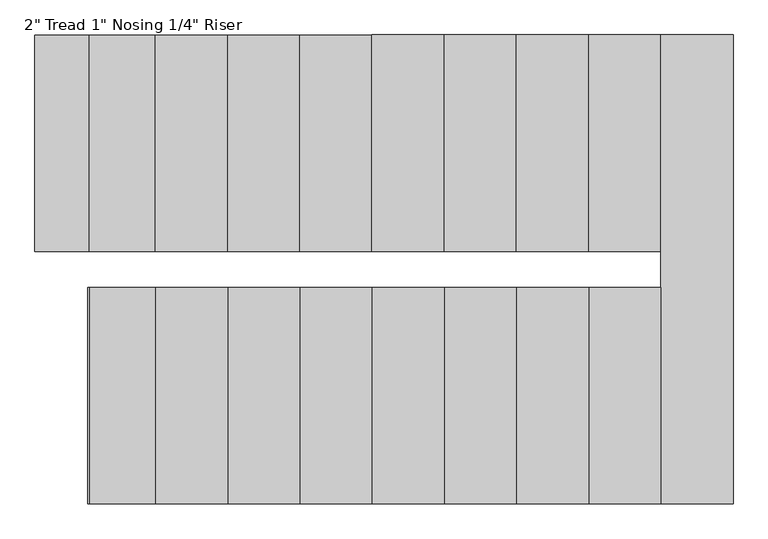
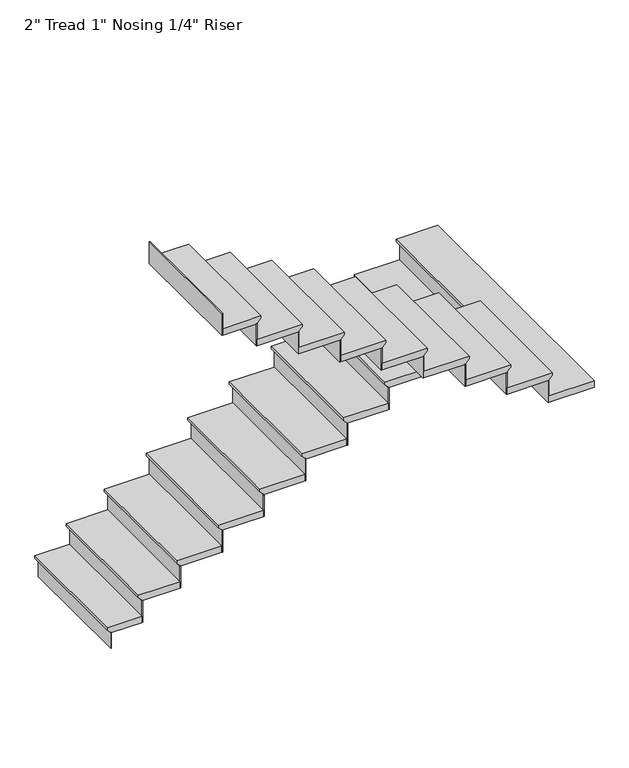
"""IFC4 building model written with IfcOpenShell, lengths in millimetres: stair flight geometry."""

from ifc_helpers import new_model, si_unit, origin, place, context, project, spatial, faceted_brep, source, transform, mapped, element, save


def stair_flight_fa6bf0c5(model_context):
    return source(origin(), model_context, "Body", "Brep", [
        faceted_brep([(8572.5, 8280.4, 150.2833333), (8572.5, 8280.4, 169.3333333), (8572.5, 9194.8, 169.3333333), (8572.5, 9194.8, 150.2833333), (8597.9, 8280.4, 124.8833333), (8597.9, 9194.8, 124.8833333), (8826.5, 8280.4, 169.3333333), (8826.5, 9194.8, 169.3333333), (8597.9, 9194.8, 118.5333333), (8826.5, 9194.8, 118.5333333), (8826.5, 8280.4, 118.5333333), (8597.9, 8280.4, 118.5333333)], [[[0, 1, 2, 3]], [[4, 0, 3, 5]], [[2, 1, 6, 7]], [[8, 9, 10, 11]], [[2, 7, 9, 8, 5, 3]], [[8, 11, 4, 5]], [[6, 1, 0, 4, 11, 10]], [[7, 6, 10, 9]]]),
        faceted_brep([(8597.9, 8280.4, 118.5333333), (8597.9, 8280.4, 0.0), (8604.25, 8280.4, 0.0), (8604.25, 8280.4, 118.5333333), (8597.9, 9194.8, 118.5333333), (8604.25, 9194.8, 118.5333333), (8604.25, 9194.8, 0.0), (8597.9, 9194.8, 0.0)], [[[0, 1, 2, 3]], [[4, 5, 6, 7]], [[1, 0, 4, 7]], [[2, 1, 7, 6]], [[3, 2, 6, 5]], [[0, 3, 5, 4]]]),
        faceted_brep([(8826.5, 8280.4, 287.8666667), (8826.5, 8280.4, 118.5333333), (8832.85, 8280.4, 118.5333333), (8832.85, 8280.4, 287.8666667), (8826.5, 9194.8, 287.8666667), (8832.85, 9194.8, 287.8666667), (8832.85, 9194.8, 118.5333333), (8826.5, 9194.8, 118.5333333)], [[[0, 1, 2, 3]], [[4, 5, 6, 7]], [[1, 0, 4, 7]], [[2, 1, 7, 6]], [[3, 2, 6, 5]], [[0, 3, 5, 4]]]),
        faceted_brep([(8801.1, 9194.8, 338.6666667), (8801.1, 8280.4, 338.6666667), (9105.9, 8280.4, 338.6666667), (9105.9, 9194.8, 338.6666667), (8826.5, 9194.8, 287.8666667), (9105.9, 9194.8, 287.8666667), (9105.9, 8280.4, 287.8666667), (8826.5, 8280.4, 287.8666667), (8826.5, 9194.8, 294.2166667), (8801.1, 9194.8, 319.6166667), (8826.5, 8280.4, 294.2166667), (8801.1, 8280.4, 319.6166667)], [[[0, 1, 2, 3]], [[4, 5, 6, 7]], [[0, 3, 5, 4, 8, 9]], [[4, 7, 10, 8]], [[2, 1, 11, 10, 7, 6]], [[3, 2, 6, 5]], [[11, 1, 0, 9]], [[10, 11, 9, 8]]]),
        faceted_brep([(9105.9, 8280.4, 457.2), (9105.9, 8280.4, 287.8666667), (9112.25, 8280.4, 287.8666667), (9112.25, 8280.4, 457.2), (9105.9, 9194.8, 457.2), (9112.25, 9194.8, 457.2), (9112.25, 9194.8, 287.8666667), (9105.9, 9194.8, 287.8666667)], [[[0, 1, 2, 3]], [[4, 5, 6, 7]], [[1, 0, 4, 7]], [[2, 1, 7, 6]], [[3, 2, 6, 5]], [[0, 3, 5, 4]]]),
        faceted_brep([(9080.5, 9194.8, 508.0), (9080.5, 8280.4, 508.0), (9410.7, 8280.4, 508.0), (9410.7, 9194.8, 508.0), (9105.9, 9194.8, 457.2), (9410.7, 9194.8, 457.2), (9410.7, 8280.4, 457.2), (9105.9, 8280.4, 457.2), (9105.9, 9194.8, 463.55), (9080.5, 9194.8, 488.95), (9105.9, 8280.4, 463.55), (9080.5, 8280.4, 488.95)], [[[0, 1, 2, 3]], [[4, 5, 6, 7]], [[0, 3, 5, 4, 8, 9]], [[4, 7, 10, 8]], [[2, 1, 11, 10, 7, 6]], [[3, 2, 6, 5]], [[11, 1, 0, 9]], [[10, 11, 9, 8]]]),
        faceted_brep([(9410.7, 8280.4, 626.5333333), (9410.7, 8280.4, 457.2), (9417.05, 8280.4, 457.2), (9417.05, 8280.4, 626.5333333), (9410.7, 9194.8, 626.5333333), (9417.05, 9194.8, 626.5333333), (9417.05, 9194.8, 457.2), (9410.7, 9194.8, 457.2)], [[[0, 1, 2, 3]], [[4, 5, 6, 7]], [[1, 0, 4, 7]], [[2, 1, 7, 6]], [[3, 2, 6, 5]], [[0, 3, 5, 4]]]),
        faceted_brep([(9385.3, 9194.8, 677.3333333), (9385.3, 8280.4, 677.3333333), (9715.5, 8280.4, 677.3333333), (9715.5, 9194.8, 677.3333333), (9410.7, 9194.8, 626.5333333), (9715.5, 9194.8, 626.5333333), (9715.5, 8280.4, 626.5333333), (9410.7, 8280.4, 626.5333333), (9410.7, 9194.8, 632.8833333), (9385.3, 9194.8, 658.2833333), (9410.7, 8280.4, 632.8833333), (9385.3, 8280.4, 658.2833333)], [[[0, 1, 2, 3]], [[4, 5, 6, 7]], [[0, 3, 5, 4, 8, 9]], [[4, 7, 10, 8]], [[2, 1, 11, 10, 7, 6]], [[3, 2, 6, 5]], [[11, 1, 0, 9]], [[10, 11, 9, 8]]]),
        faceted_brep([(9715.5, 8280.4, 795.8666667), (9715.5, 8280.4, 626.5333333), (9721.85, 8280.4, 626.5333333), (9721.85, 8280.4, 795.8666667), (9715.5, 9194.8, 795.8666667), (9721.85, 9194.8, 795.8666667), (9721.85, 9194.8, 626.5333333), (9715.5, 9194.8, 626.5333333)], [[[0, 1, 2, 3]], [[4, 5, 6, 7]], [[1, 0, 4, 7]], [[2, 1, 7, 6]], [[3, 2, 6, 5]], [[0, 3, 5, 4]]]),
        faceted_brep([(9690.1, 9194.8, 846.6666667), (9690.1, 8280.4, 846.6666667), (10020.3, 8280.4, 846.6666667), (10020.3, 9194.8, 846.6666667), (9715.5, 9194.8, 795.8666667), (10020.3, 9194.8, 795.8666667), (10020.3, 8280.4, 795.8666667), (9715.5, 8280.4, 795.8666667), (9715.5, 9194.8, 802.2166667), (9690.1, 9194.8, 827.6166667), (9715.5, 8280.4, 802.2166667), (9690.1, 8280.4, 827.6166667)], [[[0, 1, 2, 3]], [[4, 5, 6, 7]], [[0, 3, 5, 4, 8, 9]], [[4, 7, 10, 8]], [[2, 1, 11, 10, 7, 6]], [[3, 2, 6, 5]], [[11, 1, 0, 9]], [[10, 11, 9, 8]]]),
        faceted_brep([(10020.3, 8280.4, 965.2), (10020.3, 8280.4, 795.8666667), (10026.65, 8280.4, 795.8666667), (10026.65, 8280.4, 965.2), (10020.3, 9194.8, 965.2), (10026.65, 9194.8, 965.2), (10026.65, 9194.8, 795.8666667), (10020.3, 9194.8, 795.8666667)], [[[0, 1, 2, 3]], [[4, 5, 6, 7]], [[1, 0, 4, 7]], [[2, 1, 7, 6]], [[3, 2, 6, 5]], [[0, 3, 5, 4]]]),
        faceted_brep([(9994.9, 9194.8, 1016.0), (9994.9, 8280.4, 1016.0), (10325.1, 8280.4, 1016.0), (10325.1, 9194.8, 1016.0), (10020.3, 9194.8, 965.2), (10325.1, 9194.8, 965.2), (10325.1, 8280.4, 965.2), (10020.3, 8280.4, 965.2), (10020.3, 9194.8, 971.55), (9994.9, 9194.8, 996.95), (10020.3, 8280.4, 971.55), (9994.9, 8280.4, 996.95)], [[[0, 1, 2, 3]], [[4, 5, 6, 7]], [[0, 3, 5, 4, 8, 9]], [[4, 7, 10, 8]], [[2, 1, 11, 10, 7, 6]], [[3, 2, 6, 5]], [[11, 1, 0, 9]], [[10, 11, 9, 8]]]),
        faceted_brep([(10325.1, 8280.4, 1134.5333333), (10325.1, 8280.4, 965.2), (10331.45, 8280.4, 965.2), (10331.45, 8280.4, 1134.5333333), (10325.1, 9194.8, 1134.5333333), (10331.45, 9194.8, 1134.5333333), (10331.45, 9194.8, 965.2), (10325.1, 9194.8, 965.2)], [[[0, 1, 2, 3]], [[4, 5, 6, 7]], [[1, 0, 4, 7]], [[2, 1, 7, 6]], [[3, 2, 6, 5]], [[0, 3, 5, 4]]]),
        faceted_brep([(10299.7, 9194.8, 1185.3333333), (10299.7, 8280.4, 1185.3333333), (10629.9, 8280.4, 1185.3333333), (10629.9, 9194.8, 1185.3333333), (10325.1, 9194.8, 1134.5333333), (10629.9, 9194.8, 1134.5333333), (10629.9, 8280.4, 1134.5333333), (10325.1, 8280.4, 1134.5333333), (10325.1, 9194.8, 1140.8833333), (10299.7, 9194.8, 1166.2833333), (10325.1, 8280.4, 1140.8833333), (10299.7, 8280.4, 1166.2833333)], [[[0, 1, 2, 3]], [[4, 5, 6, 7]], [[0, 3, 5, 4, 8, 9]], [[4, 7, 10, 8]], [[2, 1, 11, 10, 7, 6]], [[3, 2, 6, 5]], [[11, 1, 0, 9]], [[10, 11, 9, 8]]]),
        faceted_brep([(10629.9, 8280.4, 1303.8666667), (10629.9, 8280.4, 1134.5333333), (10636.25, 8280.4, 1134.5333333), (10636.25, 8280.4, 1303.8666667), (10629.9, 9194.8, 1303.8666667), (10636.25, 9194.8, 1303.8666667), (10636.25, 9194.8, 1134.5333333), (10629.9, 9194.8, 1134.5333333)], [[[0, 1, 2, 3]], [[4, 5, 6, 7]], [[1, 0, 4, 7]], [[2, 1, 7, 6]], [[3, 2, 6, 5]], [[0, 3, 5, 4]]]),
        faceted_brep([(10604.5, 9194.8, 1354.6666667), (10604.5, 8280.4, 1354.6666667), (10934.7, 8280.4, 1354.6666667), (10934.7, 9194.8, 1354.6666667), (10629.9, 9194.8, 1303.8666667), (10934.7, 9194.8, 1303.8666667), (10934.7, 8280.4, 1303.8666667), (10629.9, 8280.4, 1303.8666667), (10629.9, 9194.8, 1310.2166667), (10604.5, 9194.8, 1335.6166667), (10629.9, 8280.4, 1310.2166667), (10604.5, 8280.4, 1335.6166667)], [[[0, 1, 2, 3]], [[4, 5, 6, 7]], [[0, 3, 5, 4, 8, 9]], [[4, 7, 10, 8]], [[2, 1, 11, 10, 7, 6]], [[3, 2, 6, 5]], [[11, 1, 0, 9]], [[10, 11, 9, 8]]]),
        faceted_brep([(10934.7, 8280.4, 1473.2), (10934.7, 8280.4, 1303.8666667), (10941.05, 8280.4, 1303.8666667), (10941.05, 8280.4, 1473.2), (10934.7, 9194.8, 1473.2), (10941.05, 9194.8, 1473.2), (10941.05, 9194.8, 1303.8666667), (10934.7, 9194.8, 1303.8666667)], [[[0, 1, 2, 3]], [[4, 5, 6, 7]], [[1, 0, 4, 7]], [[2, 1, 7, 6]], [[3, 2, 6, 5]], [[0, 3, 5, 4]]]),
        faceted_brep([(10909.3, 9194.8, 1524.0), (10909.3, 8280.4, 1524.0), (11239.5, 8280.4, 1524.0), (11239.5, 9194.8, 1524.0), (10934.7, 9194.8, 1473.2), (11239.5, 9194.8, 1473.2), (11239.5, 8280.4, 1473.2), (10934.7, 8280.4, 1473.2), (10934.7, 9194.8, 1479.55), (10909.3, 9194.8, 1504.95), (10934.7, 8280.4, 1479.55), (10909.3, 8280.4, 1504.95)], [[[0, 1, 2, 3]], [[4, 5, 6, 7]], [[0, 3, 5, 4, 8, 9]], [[4, 7, 10, 8]], [[2, 1, 11, 10, 7, 6]], [[3, 2, 6, 5]], [[11, 1, 0, 9]], [[10, 11, 9, 8]]]),
        faceted_brep([(11239.5, 8280.4, 1642.5333333), (11239.5, 8280.4, 1473.2), (11245.85, 8280.4, 1473.2), (11245.85, 8280.4, 1642.5333333), (11239.5, 9194.8, 1642.5333333), (11245.85, 9194.8, 1642.5333333), (11245.85, 9194.8, 1473.2), (11239.5, 9194.8, 1473.2)], [[[0, 1, 2, 3]], [[4, 5, 6, 7]], [[1, 0, 4, 7]], [[2, 1, 7, 6]], [[3, 2, 6, 5]], [[0, 3, 5, 4]]]),
        faceted_brep([(11188.7, 7213.6, 1693.3333333), (11518.9, 7213.6, 1693.3333333), (11518.9, 9194.8, 1693.3333333), (11214.1, 9194.8, 1693.3333333), (11214.1, 8128.0, 1693.3333333), (11188.7, 8128.0, 1693.3333333), (11518.9, 7213.6, 1642.5333333), (11188.7, 7213.6, 1642.5333333), (11188.7, 8128.0, 1642.5333333), (11214.1, 8128.0, 1642.5333333), (11214.1, 8280.4, 1642.5333333), (11239.5, 8280.4, 1642.5333333), (11239.5, 9194.8, 1642.5333333), (11518.9, 9194.8, 1642.5333333), (11239.5, 9194.8, 1648.8833333), (11214.1, 9194.8, 1674.2833333), (11239.5, 8280.4, 1648.8833333), (11214.1, 8280.4, 1674.2833333)], [[[0, 1, 2, 3, 4, 5]], [[6, 7, 8, 9, 10, 11, 12, 13]], [[1, 0, 7, 6]], [[2, 1, 6, 13]], [[3, 2, 13, 12, 14, 15]], [[12, 11, 16, 14]], [[11, 10, 17, 16]], [[4, 3, 15, 17, 10, 9]], [[5, 4, 9, 8]], [[0, 5, 8, 7]], [[15, 14, 16, 17]]]),
        faceted_brep([(11188.7, 8128.0, 1811.8666667), (11188.7, 8128.0, 1642.5333333), (11182.35, 8128.0, 1642.5333333), (11182.35, 8128.0, 1811.8666667), (11188.7, 7213.6, 1811.8666667), (11182.35, 7213.6, 1811.8666667), (11182.35, 7213.6, 1642.5333333), (11188.7, 7213.6, 1642.5333333)], [[[0, 1, 2, 3]], [[4, 5, 6, 7]], [[1, 0, 4, 7]], [[2, 1, 7, 6]], [[3, 2, 6, 5]], [[0, 3, 5, 4]]]),
        faceted_brep([(11214.1, 7213.6, 1862.6666667), (11214.1, 8128.0, 1862.6666667), (10883.9, 8128.0, 1862.6666667), (10883.9, 7213.6, 1862.6666667), (11188.7, 7213.6, 1811.8666667), (10883.9, 7213.6, 1811.8666667), (10883.9, 8128.0, 1811.8666667), (11188.7, 8128.0, 1811.8666667), (11188.7, 7213.6, 1818.2166667), (11214.1, 7213.6, 1843.6166667), (11188.7, 8128.0, 1818.2166667), (11214.1, 8128.0, 1843.6166667)], [[[0, 1, 2, 3]], [[4, 5, 6, 7]], [[0, 3, 5, 4, 8, 9]], [[4, 7, 10, 8]], [[2, 1, 11, 10, 7, 6]], [[3, 2, 6, 5]], [[11, 1, 0, 9]], [[10, 11, 9, 8]]]),
        faceted_brep([(10883.9, 8128.0, 1981.2), (10883.9, 8128.0, 1811.8666667), (10877.55, 8128.0, 1811.8666667), (10877.55, 8128.0, 1981.2), (10883.9, 7213.6, 1981.2), (10877.55, 7213.6, 1981.2), (10877.55, 7213.6, 1811.8666667), (10883.9, 7213.6, 1811.8666667)], [[[0, 1, 2, 3]], [[4, 5, 6, 7]], [[1, 0, 4, 7]], [[2, 1, 7, 6]], [[3, 2, 6, 5]], [[0, 3, 5, 4]]]),
        faceted_brep([(10909.3, 7213.6, 2032.0), (10909.3, 8128.0, 2032.0), (10579.1, 8128.0, 2032.0), (10579.1, 7213.6, 2032.0), (10883.9, 7213.6, 1981.2), (10579.1, 7213.6, 1981.2), (10579.1, 8128.0, 1981.2), (10883.9, 8128.0, 1981.2), (10883.9, 7213.6, 1987.55), (10909.3, 7213.6, 2012.95), (10883.9, 8128.0, 1987.55), (10909.3, 8128.0, 2012.95)], [[[0, 1, 2, 3]], [[4, 5, 6, 7]], [[0, 3, 5, 4, 8, 9]], [[4, 7, 10, 8]], [[2, 1, 11, 10, 7, 6]], [[3, 2, 6, 5]], [[11, 1, 0, 9]], [[10, 11, 9, 8]]]),
        faceted_brep([(10579.1, 8128.0, 2150.5333333), (10579.1, 8128.0, 1981.2), (10572.75, 8128.0, 1981.2), (10572.75, 8128.0, 2150.5333333), (10579.1, 7213.6, 2150.5333333), (10572.75, 7213.6, 2150.5333333), (10572.75, 7213.6, 1981.2), (10579.1, 7213.6, 1981.2)], [[[0, 1, 2, 3]], [[4, 5, 6, 7]], [[1, 0, 4, 7]], [[2, 1, 7, 6]], [[3, 2, 6, 5]], [[0, 3, 5, 4]]]),
        faceted_brep([(10604.5, 7213.6, 2201.3333333), (10604.5, 8128.0, 2201.3333333), (10274.3, 8128.0, 2201.3333333), (10274.3, 7213.6, 2201.3333333), (10579.1, 7213.6, 2150.5333333), (10274.3, 7213.6, 2150.5333333), (10274.3, 8128.0, 2150.5333333), (10579.1, 8128.0, 2150.5333333), (10579.1, 7213.6, 2156.8833333), (10604.5, 7213.6, 2182.2833333), (10579.1, 8128.0, 2156.8833333), (10604.5, 8128.0, 2182.2833333)], [[[0, 1, 2, 3]], [[4, 5, 6, 7]], [[0, 3, 5, 4, 8, 9]], [[4, 7, 10, 8]], [[2, 1, 11, 10, 7, 6]], [[3, 2, 6, 5]], [[11, 1, 0, 9]], [[10, 11, 9, 8]]]),
        faceted_brep([(10274.3, 8128.0, 2319.8666667), (10274.3, 8128.0, 2150.5333333), (10267.95, 8128.0, 2150.5333333), (10267.95, 8128.0, 2319.8666667), (10274.3, 7213.6, 2319.8666667), (10267.95, 7213.6, 2319.8666667), (10267.95, 7213.6, 2150.5333333), (10274.3, 7213.6, 2150.5333333)], [[[0, 1, 2, 3]], [[4, 5, 6, 7]], [[1, 0, 4, 7]], [[2, 1, 7, 6]], [[3, 2, 6, 5]], [[0, 3, 5, 4]]]),
        faceted_brep([(10299.7, 7213.6, 2370.6666667), (10299.7, 8128.0, 2370.6666667), (9969.5, 8128.0, 2370.6666667), (9969.5, 7213.6, 2370.6666667), (10274.3, 7213.6, 2319.8666667), (9969.5, 7213.6, 2319.8666667), (9969.5, 8128.0, 2319.8666667), (10274.3, 8128.0, 2319.8666667), (10274.3, 7213.6, 2326.2166667), (10299.7, 7213.6, 2351.6166667), (10274.3, 8128.0, 2326.2166667), (10299.7, 8128.0, 2351.6166667)], [[[0, 1, 2, 3]], [[4, 5, 6, 7]], [[0, 3, 5, 4, 8, 9]], [[4, 7, 10, 8]], [[2, 1, 11, 10, 7, 6]], [[3, 2, 6, 5]], [[11, 1, 0, 9]], [[10, 11, 9, 8]]]),
        faceted_brep([(9969.5, 8128.0, 2489.2), (9969.5, 8128.0, 2319.8666667), (9963.15, 8128.0, 2319.8666667), (9963.15, 8128.0, 2489.2), (9969.5, 7213.6, 2489.2), (9963.15, 7213.6, 2489.2), (9963.15, 7213.6, 2319.8666667), (9969.5, 7213.6, 2319.8666667)], [[[0, 1, 2, 3]], [[4, 5, 6, 7]], [[1, 0, 4, 7]], [[2, 1, 7, 6]], [[3, 2, 6, 5]], [[0, 3, 5, 4]]]),
        faceted_brep([(9994.9, 7213.6, 2540.0), (9994.9, 8128.0, 2540.0), (9664.7, 8128.0, 2540.0), (9664.7, 7213.6, 2540.0), (9969.5, 7213.6, 2489.2), (9664.7, 7213.6, 2489.2), (9664.7, 8128.0, 2489.2), (9969.5, 8128.0, 2489.2), (9969.5, 7213.6, 2495.55), (9994.9, 7213.6, 2520.95), (9969.5, 8128.0, 2495.55), (9994.9, 8128.0, 2520.95)], [[[0, 1, 2, 3]], [[4, 5, 6, 7]], [[0, 3, 5, 4, 8, 9]], [[4, 7, 10, 8]], [[2, 1, 11, 10, 7, 6]], [[3, 2, 6, 5]], [[11, 1, 0, 9]], [[10, 11, 9, 8]]]),
        faceted_brep([(9664.7, 8128.0, 2658.5333333), (9664.7, 8128.0, 2489.2), (9658.35, 8128.0, 2489.2), (9658.35, 8128.0, 2658.5333333), (9664.7, 7213.6, 2658.5333333), (9658.35, 7213.6, 2658.5333333), (9658.35, 7213.6, 2489.2), (9664.7, 7213.6, 2489.2)], [[[0, 1, 2, 3]], [[4, 5, 6, 7]], [[1, 0, 4, 7]], [[2, 1, 7, 6]], [[3, 2, 6, 5]], [[0, 3, 5, 4]]]),
        faceted_brep([(9690.1, 7213.6, 2709.3333333), (9690.1, 8128.0, 2709.3333333), (9359.9, 8128.0, 2709.3333333), (9359.9, 7213.6, 2709.3333333), (9664.7, 7213.6, 2658.5333333), (9359.9, 7213.6, 2658.5333333), (9359.9, 8128.0, 2658.5333333), (9664.7, 8128.0, 2658.5333333), (9664.7, 7213.6, 2664.8833333), (9690.1, 7213.6, 2690.2833333), (9664.7, 8128.0, 2664.8833333), (9690.1, 8128.0, 2690.2833333)], [[[0, 1, 2, 3]], [[4, 5, 6, 7]], [[0, 3, 5, 4, 8, 9]], [[4, 7, 10, 8]], [[2, 1, 11, 10, 7, 6]], [[3, 2, 6, 5]], [[11, 1, 0, 9]], [[10, 11, 9, 8]]]),
        faceted_brep([(9359.9, 8128.0, 2827.8666667), (9359.9, 8128.0, 2658.5333333), (9353.55, 8128.0, 2658.5333333), (9353.55, 8128.0, 2827.8666667), (9359.9, 7213.6, 2827.8666667), (9353.55, 7213.6, 2827.8666667), (9353.55, 7213.6, 2658.5333333), (9359.9, 7213.6, 2658.5333333)], [[[0, 1, 2, 3]], [[4, 5, 6, 7]], [[1, 0, 4, 7]], [[2, 1, 7, 6]], [[3, 2, 6, 5]], [[0, 3, 5, 4]]]),
        faceted_brep([(9385.3, 7213.6, 2878.6666667), (9385.3, 8128.0, 2878.6666667), (9055.1, 8128.0, 2878.6666667), (9055.1, 7213.6, 2878.6666667), (9359.9, 7213.6, 2827.8666667), (9055.1, 7213.6, 2827.8666667), (9055.1, 8128.0, 2827.8666667), (9359.9, 8128.0, 2827.8666667), (9359.9, 7213.6, 2834.2166667), (9385.3, 7213.6, 2859.6166667), (9359.9, 8128.0, 2834.2166667), (9385.3, 8128.0, 2859.6166667)], [[[0, 1, 2, 3]], [[4, 5, 6, 7]], [[0, 3, 5, 4, 8, 9]], [[4, 7, 10, 8]], [[2, 1, 11, 10, 7, 6]], [[3, 2, 6, 5]], [[11, 1, 0, 9]], [[10, 11, 9, 8]]]),
        faceted_brep([(9055.1, 8128.0, 2997.2), (9055.1, 8128.0, 2827.8666667), (9048.75, 8128.0, 2827.8666667), (9048.75, 8128.0, 2997.2), (9055.1, 7213.6, 2997.2), (9048.75, 7213.6, 2997.2), (9048.75, 7213.6, 2827.8666667), (9055.1, 7213.6, 2827.8666667)], [[[0, 1, 2, 3]], [[4, 5, 6, 7]], [[1, 0, 4, 7]], [[2, 1, 7, 6]], [[3, 2, 6, 5]], [[0, 3, 5, 4]]]),
        faceted_brep([(8801.1, 8128.0, 3166.5333333), (8801.1, 8128.0, 2997.2), (8794.75, 8128.0, 2997.2), (8794.75, 8128.0, 3166.5333333), (8801.1, 7213.6, 3166.5333333), (8794.75, 7213.6, 3166.5333333), (8794.75, 7213.6, 2997.2), (8801.1, 7213.6, 2997.2)], [[[0, 1, 2, 3]], [[4, 5, 6, 7]], [[1, 0, 4, 7]], [[2, 1, 7, 6]], [[3, 2, 6, 5]], [[0, 3, 5, 4]]]),
        faceted_brep([(9080.5, 7213.6, 3048.0), (9080.5, 8128.0, 3048.0), (8801.1, 8128.0, 3048.0), (8801.1, 7213.6, 3048.0), (9055.1, 7213.6, 2997.2), (8801.1, 7213.6, 2997.2), (8801.1, 8128.0, 2997.2), (9055.1, 8128.0, 2997.2), (9055.1, 7213.6, 3003.55), (9080.5, 7213.6, 3028.95), (9055.1, 8128.0, 3003.55), (9080.5, 8128.0, 3028.95)], [[[0, 1, 2, 3]], [[4, 5, 6, 7]], [[0, 3, 5, 4, 8, 9]], [[4, 7, 10, 8]], [[2, 1, 11, 10, 7, 6]], [[3, 2, 6, 5]], [[11, 1, 0, 9]], [[10, 11, 9, 8]]]),
    ])


if __name__ == "__main__":
    model = new_model("IFC4")
    model_context = context("Model", 3, world=origin())
    ifc_project = project(units=[si_unit("LENGTHUNIT", "METRE", prefix="MILLI")], contexts=[model_context])
    site = spatial("IfcSite", under=ifc_project)
    building = spatial("IfcBuilding", under=site)
    placement = place(None, origin())
    stair_flight_shape = stair_flight_fa6bf0c5(model_context)
    element("IfcStairFlight", 1, ObjectType="2\" Tread 1\" Nosing 1/4\" Riser", at=placement, inside=building, context=model_context, shape_type="MappedRepresentation", body=[
        mapped(stair_flight_shape, transform((0.0, 0.0, 0.0), x_axis=(1.0, 0.0, 0.0), y_axis=(0.0, 1.0, 0.0), z_axis=(0.0, 0.0, 1.0))),
    ])
    save(model, "model.ifc")
